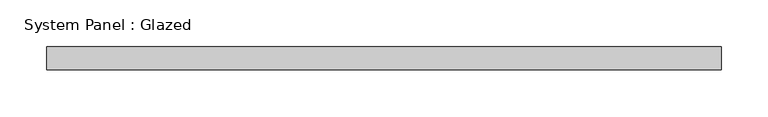
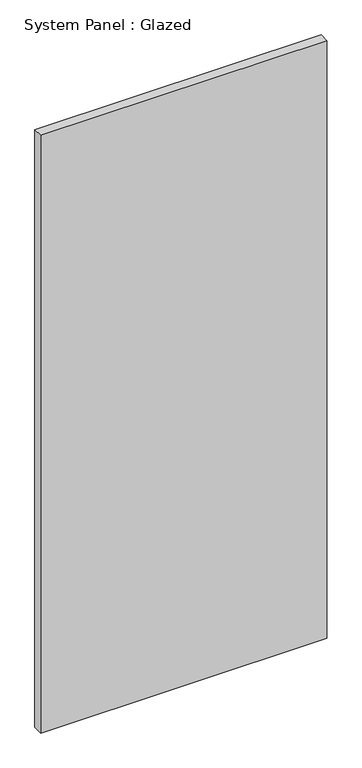
"""IFC4 building model written with IfcOpenShell, lengths in millimetres: plate geometry, System Panel : Glazed."""

from ifc_helpers import new_model, si_unit, origin, origin_with_axes, place, context, project, spatial, polyline, outline, extrude, source, transform, mapped, element, save


def system_panel_glazed_41825f56(model_context):
    return source(origin(), model_context, "Body", "SweptSolid", [
        extrude(outline(polyline([(362.5, 24.5), (-362.5, 24.5), (-362.5, 49.5), (362.5, 49.5), (362.5, 24.5)])), origin_with_axes(), (0.0, 0.0, 1.0), 1600.0),
    ])


if __name__ == "__main__":
    model = new_model("IFC4")
    model_context = context("Model", 3, world=origin())
    ifc_project = project(units=[si_unit("LENGTHUNIT", "METRE", prefix="MILLI")], contexts=[model_context])
    site = spatial("IfcSite", under=ifc_project)
    building = spatial("IfcBuilding", under=site)
    placement = place(None, origin())
    system_panel_glazed_shape = system_panel_glazed_41825f56(model_context)
    element("IfcPlate", 1, ObjectType="System Panel : Glazed", at=placement, inside=building, context=model_context, shape_type="MappedRepresentation", body=[
        mapped(system_panel_glazed_shape, transform((0.0, 0.0, 0.0), x_axis=(1.0, 0.0, 0.0), y_axis=(0.0, 1.0, 0.0), z_axis=(0.0, 0.0, 1.0))),
    ])
    save(model, "model.ifc")

# Revit data of these elements
# Type "System Panel : Glazed"
#   Construction Type Id = "GSP4R"
#   Analytic Construction = "1/8 in Pilkington single glazing"
#   Visual Light Transmittance = 0.9
#   Solar Heat Gain Coefficient = 0.86
#   Heat Transfer Coefficient (U) = 6.7069 W/(m²·K)
#   Define Thermal Properties by = 1
# Element 1 (IfcPlate, "System Panel : Glazed")
#   Materials on its faces: "Glass"
# Materials
#   "Glass": class "Glass", colour RGB 245 245 243, transparency 1, Description = "Soda Lime Glass", Cost = 0
